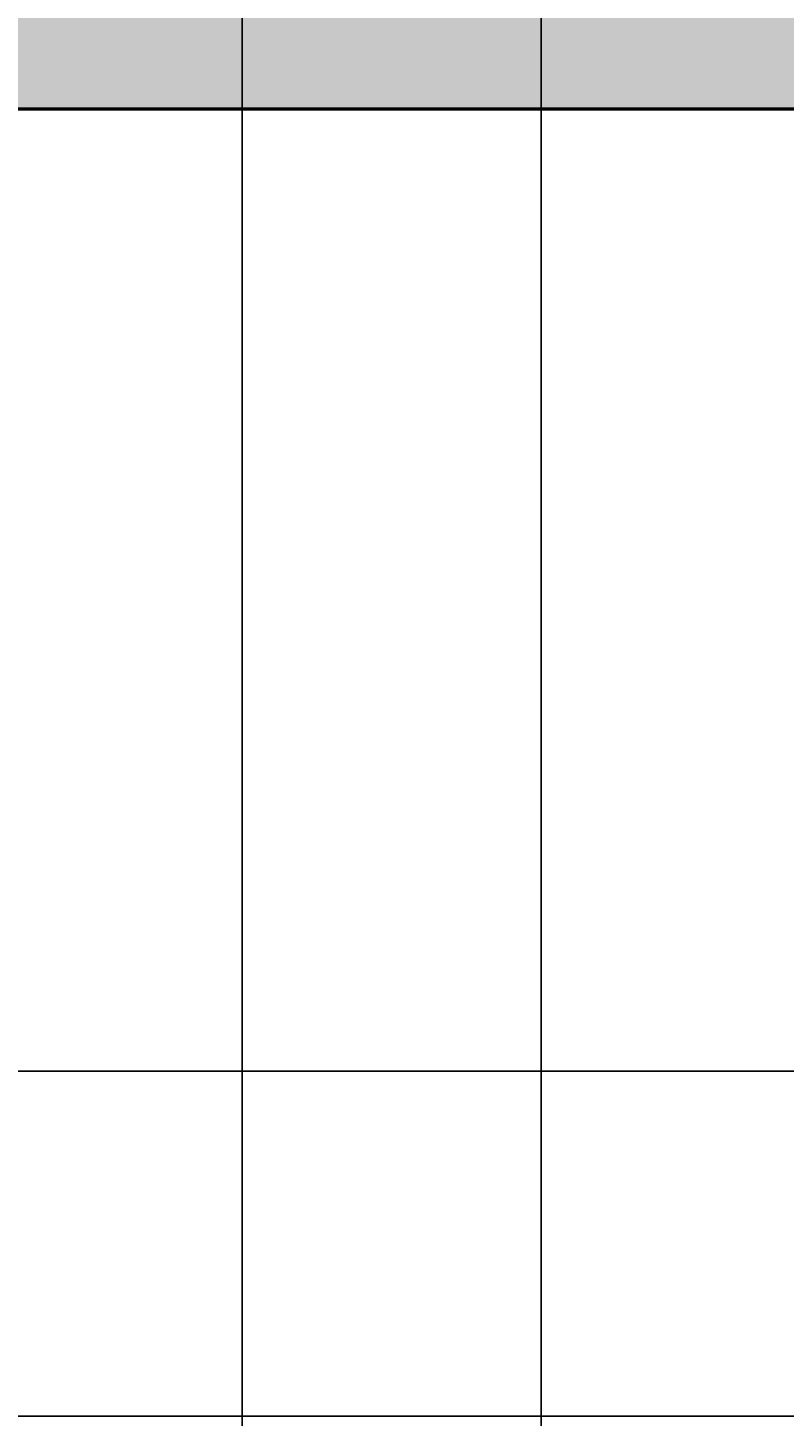
# Model space of a CAD drawing. Units: inches. Extents: x 2231 to 2461, y 2045 to 2455.
# Tile 33 of 95: x 2396 to 2415, y 2151 to 2185. Entities that reach past the tile are written whole.
import ezdxf

# ---------------------------------------------------------------- set-up
doc = ezdxf.new("R2010")
doc.units = ezdxf.units.IN
for name, color, linetype, lineweight in [('A-ANNO-DIMS', 2, 'Continuous', 18), ('A-FLOR-CASE', 8, 'Continuous', 25), ('A-WALL', 7, 'Continuous', 50)]:
    doc.layers.add(name, color=color, linetype=linetype, lineweight=lineweight)
doc.layers.add('A-WALL-PATT', color=18, linetype='Continuous', lineweight=13, true_color=0x000000)
doc.styles.get("Standard").update_dxf_attribs({"font": 'arial.ttf'})
doc.dimstyles.get("Standard").update_dxf_attribs({"dimtxt": 0.18, "dimasz": 0.18, "dimexe": 0.18, "dimexo": 0.0625, "dimgap": 0.09, "dimtad": 0, "dimtih": 1, "dimtoh": 1, "dimdec": 4, "dimzin": 0, "dimdsep": 46, "dimtxsty": 'Standard', "dimcen": 0.09, "dimadec": 0, "dimazin": 0, "dimtfac": 1, "dimtdec": 4, "dimtofl": 0, "dimtmove": 0, "dimatfit": 3, "dimfxl": 1, "dimtolj": 1, "dimtzin": 0, "dimarcsym": 0})

# ---------------------------------------------------------------- blocks, each defined once
blk = doc.blocks.new('*D59')
at = {"layer": 'A-ANNO-DIMS', "color": 0, "lineweight": -2, "transparency": 16777216}
for p, q in [((2408.794, 2182.895), (2408.794, 2454.645)), ((2432.794, 2182.895), (2432.794, 2454.645)), ((2408.974, 2454.465), (2420.573, 2454.465)), ((2432.614, 2454.465), (2421.014, 2454.465))]:
    blk.add_line(p, q, dxfattribs=at)
at = {"layer": 'A-ANNO-DIMS', "color": 0, "transparency": 16777216}
for points in [[(2408.974, 2454.495), (2408.974, 2454.435), (2408.794, 2454.465)], [(2432.614, 2454.495), (2432.614, 2454.435), (2432.794, 2454.465)]]:
    blk.add_solid(points, dxfattribs=at)
at = {"layer": 'Defpoints', "color": 0, "transparency": 16777216}
for p in [(2432.794, 2454.465), (2408.794, 2182.833), (2432.794, 2182.833)]:
    blk.add_point(p, dxfattribs=at)
at = {"layer": 'A-ANNO-DIMS', "color": 0, "transparency": 16777216, "insert": (2420.794, 2454.465), "char_height": 0.18, "attachment_point": 5}
blk.add_mtext('\\A1;24', dxfattribs=at)
blk = doc.blocks.new('*D60')
at = {"layer": 'A-ANNO-DIMS', "color": 0, "lineweight": -2, "transparency": 16777216}
for p, q in [((2432.731, 2182.833), (2230.981, 2182.833)), ((2231.161, 2182.653), (2231.161, 2166.906)), ((2231.161, 2150.795), (2231.161, 2166.542)), ((2432.731, 2150.615), (2230.981, 2150.615))]:
    blk.add_line(p, q, dxfattribs=at)
at = {"layer": 'A-ANNO-DIMS', "color": 0, "transparency": 16777216}
for points in [[(2231.131, 2182.653), (2231.191, 2182.653), (2231.161, 2182.833)], [(2231.131, 2150.795), (2231.191, 2150.795), (2231.161, 2150.615)]]:
    blk.add_solid(points, dxfattribs=at)
at = {"layer": 'Defpoints', "color": 0, "transparency": 16777216}
for p in [(2231.161, 2182.833), (2432.794, 2182.833), (2432.794, 2150.615)]:
    blk.add_point(p, dxfattribs=at)
at = {"layer": 'A-ANNO-DIMS', "color": 0, "transparency": 16777216, "insert": (2231.161, 2166.724), "char_height": 0.18, "attachment_point": 5}
blk.add_mtext('\\A1;32.22', dxfattribs=at)
blk = doc.blocks.new('*D66')
at = {"layer": 'A-ANNO-DIMS', "color": 0, "lineweight": -2, "transparency": 16777216}
for p, q in [((2348.189, 2096.895), (2348.189, 2454.645)), ((2408.794, 2096.895), (2408.794, 2454.645)), ((2348.369, 2454.465), (2378.167, 2454.465)), ((2408.614, 2454.465), (2378.815, 2454.465))]:
    blk.add_line(p, q, dxfattribs=at)
at = {"layer": 'A-ANNO-DIMS', "color": 0, "transparency": 16777216}
for points in [[(2348.369, 2454.495), (2348.369, 2454.435), (2348.189, 2454.465)], [(2408.614, 2454.495), (2408.614, 2454.435), (2408.794, 2454.465)]]:
    blk.add_solid(points, dxfattribs=at)
at = {"layer": 'Defpoints', "color": 0, "transparency": 16777216}
for p in [(2408.794, 2454.465), (2348.189, 2096.833), (2408.794, 2096.833)]:
    blk.add_point(p, dxfattribs=at)
at = {"layer": 'A-ANNO-DIMS', "color": 0, "transparency": 16777216, "insert": (2378.491, 2454.465), "char_height": 0.18, "attachment_point": 5}
blk.add_mtext('\\A1;60.6', dxfattribs=at)
blk = doc.blocks.new('*D71')
at = {"layer": 'A-ANNO-DIMS', "color": 0, "lineweight": -2, "transparency": 16777216}
for p, q in [((2401.422, 2092.979), (2401.422, 2454.645)), ((2408.794, 2096.895), (2408.794, 2454.645)), ((2401.602, 2454.465), (2404.732, 2454.465)), ((2408.614, 2454.465), (2405.483, 2454.465))]:
    blk.add_line(p, q, dxfattribs=at)
at = {"layer": 'A-ANNO-DIMS', "color": 0, "transparency": 16777216}
for points in [[(2401.602, 2454.495), (2401.602, 2454.435), (2401.422, 2454.465)], [(2408.614, 2454.495), (2408.614, 2454.435), (2408.794, 2454.465)]]:
    blk.add_solid(points, dxfattribs=at)
at = {"layer": 'Defpoints', "color": 0, "transparency": 16777216}
for p in [(2408.794, 2454.465), (2408.794, 2096.833), (2401.422, 2092.917)]:
    blk.add_point(p, dxfattribs=at)
at = {"layer": 'A-ANNO-DIMS', "color": 0, "transparency": 16777216, "insert": (2405.108, 2454.465), "char_height": 0.18, "attachment_point": 5}
blk.add_mtext('\\A1;7.371', dxfattribs=at)
blk = doc.blocks.new('*D72')
at = {"layer": 'A-ANNO-DIMS', "color": 0, "lineweight": -2, "transparency": 16777216}
for p, q in [((2384.543, 2145.12), (2384.543, 2454.645)), ((2408.794, 2150.677), (2408.794, 2454.645)), ((2384.723, 2454.465), (2396.272, 2454.465)), ((2408.614, 2454.465), (2397.064, 2454.465))]:
    blk.add_line(p, q, dxfattribs=at)
at = {"layer": 'A-ANNO-DIMS', "color": 0, "transparency": 16777216}
for points in [[(2384.723, 2454.495), (2384.723, 2454.435), (2384.543, 2454.465)], [(2408.614, 2454.495), (2408.614, 2454.435), (2408.794, 2454.465)]]:
    blk.add_solid(points, dxfattribs=at)
at = {"layer": 'Defpoints', "color": 0, "transparency": 16777216}
for p in [(2408.794, 2454.465), (2408.794, 2150.615), (2384.543, 2145.058)]:
    blk.add_point(p, dxfattribs=at)
at = {"layer": 'A-ANNO-DIMS', "color": 0, "transparency": 16777216, "insert": (2396.668, 2454.465), "char_height": 0.18, "attachment_point": 5}
blk.add_mtext('\\A1;24.25', dxfattribs=at)
blk = doc.blocks.new('*D73')
at = {"layer": 'A-ANNO-DIMS', "color": 0, "lineweight": -2, "transparency": 16777216}
for p, q in [((2334.856, 2182.833), (2460.606, 2182.833)), ((2460.426, 2182.653), (2460.426, 2171.156)), ((2460.426, 2159.295), (2460.426, 2170.792)), ((2353.872, 2159.115), (2460.606, 2159.115))]:
    blk.add_line(p, q, dxfattribs=at)
at = {"layer": 'A-ANNO-DIMS', "color": 0, "transparency": 16777216}
for points in [[(2460.396, 2182.653), (2460.456, 2182.653), (2460.426, 2182.833)], [(2460.396, 2159.295), (2460.456, 2159.295), (2460.426, 2159.115)]]:
    blk.add_solid(points, dxfattribs=at)
at = {"layer": 'Defpoints', "color": 0, "transparency": 16777216}
for p in [(2334.794, 2182.833), (2460.426, 2182.833), (2353.809, 2159.115)]:
    blk.add_point(p, dxfattribs=at)
at = {"layer": 'A-ANNO-DIMS', "color": 0, "transparency": 16777216, "insert": (2460.426, 2170.974), "char_height": 0.18, "attachment_point": 5}
blk.add_mtext('\\A1;23.717', dxfattribs=at)

msp = doc.modelspace()

# ---------------------------------------------------------------- hatches: boundary and pattern name
at = {"layer": 'A-WALL-PATT'}
h = msp.add_hatch(color=256, dxfattribs=at)
h.dxf.hatch_style = 1
h.paths.add_polyline_path([(2441.7935, 2269.1535), (2432.7935, 2269.1535), (2432.7935, 2186.8328), (2396.7935, 2186.8328), (2396.7935, 2286.8328), (2394.7935, 2286.8328), (2394.7935, 2186.8328), (2334.7935, 2186.8328), (2334.7935, 2182.8328), (2432.7935, 2182.8328), (2432.7935, 2072.8328), (2416.6639, 2072.8328), (2416.6639, 2063.8328), (2441.7935, 2063.8328)])
h.paths.add_polyline_path([(2368.6639, 2072.8328), (2367.04, 2072.8328), (2330.7942, 2072.8328), (2330.7397, 2063.8328), (2368.6639, 2063.8328)])
h.paths.add_polyline_path([(2300.7392, 2068.3328), (2300.7392, 2072.8328), (2298.7935, 2072.8328), (2294.7935, 2072.8328), (2258.7935, 2072.8328), (2258.7935, 2120.8328), (2294.7935, 2120.8328), (2298.7935, 2120.8328), (2298.7935, 2128.8328), (2294.7935, 2128.8328), (2294.7935, 2124.8328), (2258.7935, 2124.8328), (2258.7935, 2182.8328), (2294.7935, 2182.8328), (2294.7935, 2174.8328), (2298.7935, 2174.8328), (2298.7935, 2182.8328), (2304.7935, 2182.8328), (2304.7935, 2186.8328), (2258.7935, 2186.8328), (2258.7935, 2221.999), (2249.7935, 2221.999), (2249.7935, 2063.8328), (2300.7392, 2063.8328)])
h.paths.add_polyline_path([(2391.9338, 2435.8328), (2333.82, 2435.8328), (2333.82, 2426.8328), (2368.7935, 2426.8328), (2368.7935, 2374.9508), (2368.7935, 2370.8328), (2372.3935, 2370.8328), (2372.7935, 2370.8328), (2372.7935, 2426.8328), (2391.9338, 2426.8328)])
h.paths.add_polyline_path([(2441.7935, 2435.8328), (2415.9338, 2435.8328), (2415.9338, 2426.8328), (2432.7935, 2426.8328), (2432.7935, 2334.8328), (2372.7935, 2334.8328), (2372.7935, 2346.8328), (2368.7935, 2346.8328), (2368.7935, 2306.8328), (2360.7935, 2306.8328), (2360.7935, 2302.8328), (2368.7935, 2302.8328), (2372.7935, 2302.8328), (2372.7935, 2330.8328), (2432.7935, 2330.8328), (2432.7935, 2317.1535), (2441.7935, 2317.1535)])
h.paths.add_polyline_path([(2285.82, 2435.8328), (2249.7935, 2435.8328), (2249.7935, 2269.999), (2258.7935, 2269.999), (2258.7935, 2302.8328), (2318.8168, 2302.8328), (2330.7935, 2302.8328), (2330.7935, 2306.8328), (2258.7935, 2306.8328), (2258.7935, 2426.8328), (2285.82, 2426.8328)])

# ---------------------------------------------------------------- linework, layer by layer
at = {"layer": 'A-FLOR-CASE'}
msp.add_line((2408.7935, 2182.8328), (2408.7935, 2096.8328), dxfattribs=at)
at = {"layer": 'A-WALL'}
msp.add_line((2334.7935, 2182.8328), (2432.7935, 2182.8328), dxfattribs=at)

# ---------------------------------------------------------------- dimensions: what is measured, and where the dimension line sits
at = {"layer": 'A-ANNO-DIMS'}
for base, p1, p2, override, picture, middle in [((2408.7935, 2454.4653), (2348.1888, 2096.8328), (2408.7935, 2096.8328), {"dimdec": 1, "dimlfac": 1, "dimrnd": 0, "dimzin": 0, "dimdsep": 46, "dimlunit": 2}, '*D66', (2378.4912, 2454.4653)), ((2408.7935, 2454.4653), (2384.5428, 2145.0576), (2408.7935, 2150.6145), {"dimdec": 2, "dimlfac": 1, "dimrnd": 0, "dimzin": 0, "dimdsep": 46, "dimlunit": 2}, '*D72', (2396.6682, 2454.4653)), ((2408.7935, 2454.4653), (2401.4221, 2092.9167), (2408.7935, 2096.8328), {"dimdec": 3, "dimlfac": 1, "dimrnd": 0, "dimzin": 0, "dimdsep": 46, "dimlunit": 2}, '*D71', (2405.1078, 2454.4653)), ((2432.7935, 2454.4653), (2408.7935, 2182.8328), (2432.7935, 2182.8328), {"dimdec": 0, "dimlfac": 1, "dimrnd": 0, "dimzin": 0, "dimdsep": 46, "dimlunit": 2}, '*D59', (2420.7935, 2454.4653))]:
    dim = msp.add_linear_dim(base=base, p1=p1, p2=p2, dimstyle='Standard', override=override, dxfattribs=at)
    dim.commit()
    dim.dimension.update_dxf_attribs({"geometry": picture, "text_midpoint": middle})
for base, p1, p2, override, picture, middle in [((2231.161, 2182.8328), (2432.7935, 2150.6145), (2432.7935, 2182.8328), {"dimdec": 2, "dimlfac": 1, "dimrnd": 0, "dimzin": 0, "dimdsep": 46, "dimlunit": 2}, '*D60', (2231.161, 2166.7237)), ((2460.426, 2182.8328), (2353.8091, 2159.1154), (2334.7935, 2182.8328), {"dimdec": 3, "dimlfac": 1, "dimrnd": 0, "dimzin": 0, "dimdsep": 46, "dimlunit": 2}, '*D73', (2460.426, 2170.9741))]:
    dim = msp.add_linear_dim(base=base, p1=p1, p2=p2, angle=90, dimstyle='Standard', override=override, dxfattribs=at)
    dim.commit()
    dim.dimension.update_dxf_attribs({"geometry": picture, "text_midpoint": middle})

doc.saveas('drawing.dxf')
